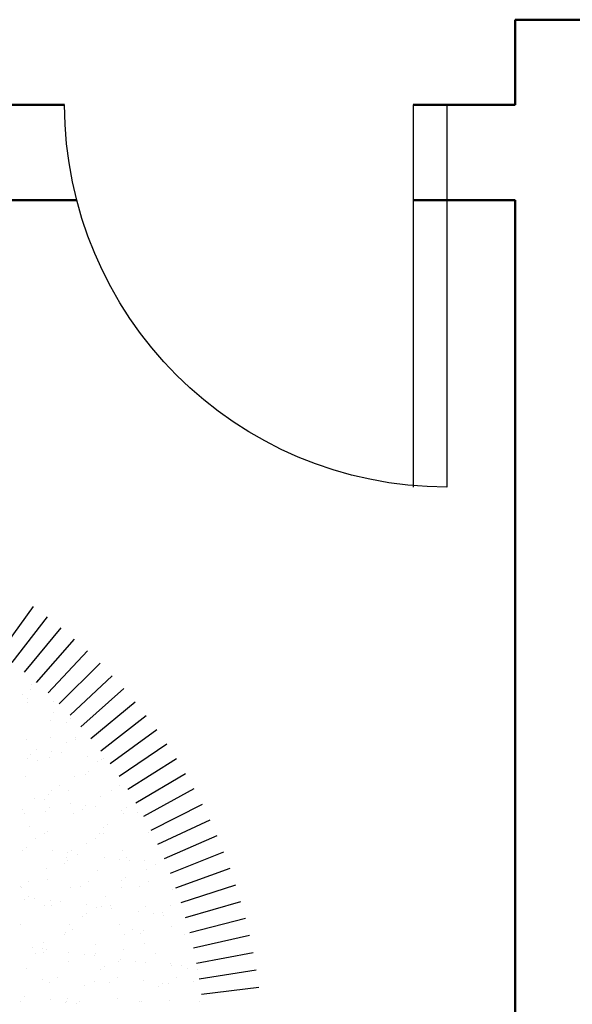
# Model space of a CAD drawing. Units: millimetres. Extents: x -857 to 54106, y -13666 to 13947.
# Tile 16 of 41: x 23479 to 24780, y 5837 to 8154. Entities that reach past the tile are written whole.
import ezdxf

# ---------------------------------------------------------------- set-up
doc = ezdxf.new("R2010")
doc.units = ezdxf.units.MM
for name, color, linetype, lineweight in [('A-DOOR', 1, 'Continuous', 25), ('A-FURN', 21, 'Continuous', 18), ('A-WALL', 7, 'Continuous', 50)]:
    doc.layers.add(name, color=color, linetype=linetype, lineweight=lineweight)
doc.layers.add('A-HT', color=15, linetype='Continuous')

# ---------------------------------------------------------------- blocks, each defined once
blk = doc.blocks.new('*X18')
at = {"color": 0}
for p, q in [((1.1527, 2.5197), (1.1527, 2.5197)), ((1.1551, 2.5078), (1.1551, 2.5078)), ((1.1761, 2.4943), (1.1761, 2.4943)), ((1.0951, 2.4744), (1.0951, 2.4744)), ((1.163, 2.4833), (1.163, 2.4833)), ((1.163, 2.4726), (1.163, 2.4726)), ((1.0963, 2.4457), (1.0963, 2.4457)), ((1.0521, 2.4302), (1.0521, 2.4302)), ((1.0613, 2.4218), (1.0613, 2.4218)), ((1.1027, 2.4263), (1.1027, 2.4263)), ((1.0383, 2.3768), (1.0383, 2.3768)), ((1.0397, 2.3823), (1.0397, 2.3823)), ((1.0608, 2.3689), (1.0608, 2.3689)), ((1.1048, 2.3819), (1.1048, 2.3819)), ((1.1662, 2.3762), (1.1662, 2.3762)), ((1.0745, 2.3422), (1.0745, 2.3422)), ((1.1005, 2.3457), (1.1005, 2.3457)), ((1.1412, 2.351), (1.1412, 2.351)), ((1.1546, 2.3363), (1.1546, 2.3363)), ((0.966, 2.3279), (0.966, 2.3279)), ((0.9708, 2.3251), (0.9708, 2.3251)), ((0.981, 2.3202), (0.981, 2.3202)), ((1.0066, 2.3333), (1.0066, 2.3333)), ((1.1059, 2.33), (1.1059, 2.33)), ((1.1367, 2.3205), (1.1367, 2.3205)), ((1.1638, 2.3279), (1.1638, 2.3279)), ((1.0043, 2.2924), (1.0043, 2.2924)), ((1.0135, 2.284), (1.0135, 2.284)), ((0.9244, 2.2568), (0.9244, 2.2568)), ((1.0414, 2.2805), (1.0414, 2.2805)), ((1.0801, 2.2571), (1.0801, 2.2571)), ((1.1693, 2.2799), (1.1693, 2.2799)), ((0.9455, 2.2434), (0.9455, 2.2434)), ((1.057, 2.2441), (1.057, 2.2441)), ((1.1012, 2.2437), (1.1012, 2.2437)), ((1.109, 2.2336), (1.109, 2.2336)), ((0.974, 2.2287), (0.974, 2.2287)), ((1.0527, 2.2099), (1.0527, 2.2099)), ((1.1206, 2.2189), (1.1206, 2.2189)), ((1.1466, 2.2223), (1.1466, 2.2223)), ((0.8775, 2.1868), (0.8775, 2.1868)), ((0.9067, 2.2002), (0.9067, 2.2002)), ((0.9137, 2.1825), (0.9137, 2.1825)), ((0.9181, 2.1922), (0.9181, 2.1922)), ((0.986, 2.2011), (0.986, 2.2011)), ((1.0121, 2.2046), (1.0121, 2.2046)), ((1.0214, 2.195), (1.0214, 2.195)), ((1.0446, 2.1841), (1.0446, 2.1841)), ((1.1068, 2.1985), (1.1068, 2.1985)), ((1.116, 2.1901), (1.116, 2.1901)), ((1.1725, 2.1835), (1.1725, 2.1835)), ((1.1771, 2.1953), (1.1771, 2.1953)), ((0.9565, 2.1546), (0.9565, 2.1546)), ((0.8492, 2.133), (0.8492, 2.133)), ((0.9648, 2.1316), (0.9648, 2.1316)), ((0.9657, 2.1462), (0.9657, 2.1462)), ((0.9771, 2.1324), (0.9771, 2.1324)), ((1.1122, 2.1373), (1.1122, 2.1373)), ((1.1205, 2.1319), (1.1205, 2.1319)), ((1.1595, 2.1502), (1.1595, 2.1502)), ((0.9859, 2.1182), (0.9859, 2.1182)), ((1.0092, 2.1063), (1.0092, 2.1063)), ((1.1416, 2.1184), (1.1416, 2.1184)), ((0.9169, 2.0861), (0.9169, 2.0861)), ((1.0321, 2.0777), (1.0321, 2.0777)), ((1.0477, 2.0878), (1.0477, 2.0878)), ((1.0582, 2.0812), (1.0582, 2.0812)), ((1.0988, 2.0865), (1.0988, 2.0865)), ((1.1667, 2.0955), (1.1667, 2.0955)), ((1.1756, 2.0872), (1.1756, 2.0872)), ((0.8589, 2.0624), (0.8589, 2.0624)), ((0.8975, 2.06), (0.8975, 2.06)), ((0.9061, 2.0695), (0.9061, 2.0695)), ((0.9236, 2.0635), (0.9236, 2.0635)), ((0.9642, 2.0688), (0.9642, 2.0688)), ((1.059, 2.0607), (1.059, 2.0607)), ((1.0618, 2.0698), (1.0618, 2.0698)), ((1.0682, 2.0523), (1.0682, 2.0523)), ((0.8296, 2.0511), (0.8296, 2.0511)), ((0.8524, 2.0367), (0.8524, 2.0367)), ((0.9803, 2.0361), (0.9803, 2.0361)), ((1.1153, 2.0409), (1.1153, 2.0409)), ((0.8495, 2.0061), (0.8495, 2.0061)), ((0.9087, 2.0168), (0.9087, 2.0168)), ((0.9179, 2.0084), (0.9179, 2.0084)), ((1.0052, 2.0064), (1.0052, 2.0064)), ((1.1117, 2.0124), (1.1117, 2.0124)), ((1.1609, 2.0067), (1.1609, 2.0067)), ((0.785, 1.9849), (0.785, 1.9849)), ((0.8706, 1.9927), (0.8706, 1.9927)), ((0.92, 1.9898), (0.92, 1.9898)), ((1.0263, 1.993), (1.0263, 1.993)), ((1.0509, 1.9915), (1.0509, 1.9915)), ((1.1788, 1.9909), (1.1788, 1.9909)), ((1.182, 1.9932), (1.182, 1.9932)), ((0.9614, 1.9685), (0.9614, 1.9685)), ((1.0782, 1.9544), (1.0782, 1.9544)), ((1.1043, 1.9578), (1.1043, 1.9578)), ((1.1449, 1.9631), (1.1449, 1.9631)), ((1.1614, 1.9668), (1.1614, 1.9668)), ((1.1707, 1.9584), (1.1707, 1.9584)), ((0.7908, 1.944), (0.7908, 1.944)), ((0.8111, 1.9247), (0.8111, 1.9247)), ((0.8555, 1.9403), (0.8555, 1.9403)), ((0.8757, 1.9277), (0.8757, 1.9277)), ((0.9436, 1.9366), (0.9436, 1.9366)), ((0.9465, 1.9443), (0.9465, 1.9443)), ((0.9697, 1.9401), (0.9697, 1.9401)), ((0.9834, 1.9397), (0.9834, 1.9397)), ((1.0103, 1.9454), (1.0103, 1.9454)), ((1.1022, 1.9446), (1.1022, 1.9446)), ((1.1185, 1.9446), (1.1185, 1.9446)), ((0.8091, 1.9189), (0.8091, 1.9189)), ((0.8351, 1.9223), (0.8351, 1.9223)), ((1.0111, 1.9229), (1.0111, 1.9229)), ((1.0204, 1.9145), (1.0204, 1.9145)), ((0.7881, 1.8886), (0.7881, 1.8886)), ((0.8608, 1.879), (0.8608, 1.879)), ((0.8898, 1.8809), (0.8898, 1.8809)), ((0.9232, 1.8935), (0.9232, 1.8935)), ((1.0456, 1.8812), (1.0456, 1.8812)), ((1.054, 1.8951), (1.054, 1.8951)), ((1.0639, 1.8746), (1.0639, 1.8746)), ((1.1819, 1.8945), (1.1819, 1.8945)), ((0.7552, 1.8672), (0.7552, 1.8672)), ((0.8701, 1.8706), (0.8701, 1.8706)), ((0.9109, 1.8675), (0.9109, 1.8675)), ((1.0666, 1.8678), (1.0666, 1.8678)), ((1.1216, 1.8482), (1.1216, 1.8482)), ((0.8587, 1.844), (0.8587, 1.844)), ((0.9136, 1.8307), (0.9136, 1.8307)), ((0.9866, 1.8434), (0.9866, 1.8434)), ((1.0564, 1.822), (1.0564, 1.822)), ((1.1136, 1.829), (1.1136, 1.829)), ((1.1243, 1.831), (1.1243, 1.831)), ((1.1504, 1.8344), (1.1504, 1.8344)), ((0.8311, 1.8188), (0.8311, 1.8188)), ((0.8552, 1.7955), (0.8552, 1.7955)), ((0.8812, 1.799), (0.8812, 1.799)), ((0.9218, 1.8043), (0.9218, 1.8043)), ((0.9263, 1.7971), (0.9263, 1.7971)), ((0.9868, 1.8191), (0.9868, 1.8191)), ((0.9897, 1.8132), (0.9897, 1.8132)), ((1.0158, 1.8167), (1.0158, 1.8167)), ((1.0572, 1.7988), (1.0572, 1.7988)), ((1.1228, 1.8206), (1.1228, 1.8206)), ((1.1425, 1.8194), (1.1425, 1.8194)), ((0.7206, 1.7778), (0.7206, 1.7778)), ((0.7466, 1.7812), (0.7466, 1.7812)), ((0.7632, 1.7869), (0.7632, 1.7869)), ((0.7872, 1.7866), (0.7872, 1.7866)), ((0.7913, 1.7922), (0.7913, 1.7922)), ((0.9633, 1.7851), (0.9633, 1.7851)), ((0.9725, 1.7767), (0.9725, 1.7767)), ((1.1663, 1.7807), (1.1663, 1.7807)), ((0.731, 1.746), (0.731, 1.746)), ((0.7745, 1.7554), (0.7745, 1.7554)), ((0.8618, 1.7477), (0.8618, 1.7477)), ((0.9302, 1.7557), (0.9302, 1.7557)), ((0.9897, 1.747), (0.9897, 1.747)), ((1.0859, 1.756), (1.0859, 1.756)), ((1.1248, 1.7519), (1.1248, 1.7519)), ((0.7956, 1.742), (0.7956, 1.742)), ((0.813, 1.7413), (0.813, 1.7413)), ((0.8222, 1.7328), (0.8222, 1.7328)), ((0.9513, 1.7423), (0.9513, 1.7423)), ((1.016, 1.7368), (1.016, 1.7368)), ((1.107, 1.7426), (1.107, 1.7426)), ((0.7158, 1.6933), (0.7158, 1.6933)), ((0.7944, 1.6959), (0.7944, 1.6959)), ((0.8657, 1.693), (0.8657, 1.693)), ((0.8715, 1.6936), (0.8715, 1.6936)), ((0.9295, 1.7008), (0.9295, 1.7008)), ((1.0272, 1.6939), (1.0272, 1.6939)), ((1.0603, 1.7024), (1.0603, 1.7024)), ((1.0619, 1.6933), (1.0619, 1.6933)), ((1.1025, 1.6986), (1.1025, 1.6986)), ((1.1704, 1.7076), (1.1704, 1.7076)), ((1.1829, 1.6942), (1.1829, 1.6942)), ((1.0358, 1.6899), (1.0358, 1.6899)), ((1.0658, 1.6912), (1.0658, 1.6912))]:
    blk.add_line(p, q, dxfattribs=at)
blk = doc.blocks.new('A$C6796526C')
at = {"layer": 'A-HT'}
for p, q in [((0.1603, 1.2871), (0.0114, 1.2683)), ((0.166, 1.2466), (0.0179, 1.2232)), ((0.173, 1.2064), (0.0257, 1.1783)), ((0.1813, 1.1664), (0.0349, 1.1337)), ((0.1908, 1.1267), (0.0456, 1.0894)), ((0.2016, 1.0873), (0.0576, 1.0455)), ((0.2136, 1.0483), (0.071, 1.0019)), ((0.2269, 1.0096), (0.0857, 0.9588)), ((0.2413, 0.9714), (0.1018, 0.9162)), ((0.2569, 0.9337), (0.1193, 0.8741)), ((0.2737, 0.8965), (0.138, 0.8326)), ((0.2917, 0.8598), (0.158, 0.7917)), ((0.3108, 0.8237), (0.1794, 0.7515)), ((0.331, 0.7882), (0.2019, 0.7119)), ((0.3524, 0.7534), (0.2257, 0.6731)), ((0.3748, 0.7193), (0.2507, 0.635)), ((0.3983, 0.6859), (0.2769, 0.5977)), ((0.4228, 0.6532), (0.3043, 0.5613)), ((0.4483, 0.6213), (0.3328, 0.5257)), ((0.4749, 0.5903), (0.3623, 0.4911)), ((0.5023, 0.5601), (0.393, 0.4574)), ((0.5308, 0.5308), (0.4247, 0.4247)), ((0.5601, 0.5023), (0.4574, 0.393)), ((0.5903, 0.4749), (0.4911, 0.3623)), ((0.6213, 0.4483), (0.5257, 0.3328)), ((0.6532, 0.4228), (0.5613, 0.3043)), ((0.6859, 0.3983), (0.5977, 0.2769))]:
    blk.add_line(p, q, dxfattribs=at)
at = {"layer": 'A-HT', "extrusion": (0, 0, -1), "zscale": -1, "rotation": 180}
blk.add_blockref('*X18', (0.55, 3), dxfattribs=at)
blk = doc.blocks.new('DOOR-900')
blk.add_line((11417.3, 9811.5), (12317.3, 9811.5))
blk.add_arc((11417.3, 9811.5), 900, 0, 90)

msp = doc.modelspace()

# ---------------------------------------------------------------- linework, layer by layer
at = {"layer": 'A-DOOR'}
msp.add_line((24404.957, 7954.231), (24404.957, 7054.231), dxfattribs=at)
at = {"layer": 'A-WALL'}
for p, q in [((24645.079, 8154.231), (24645.079, 7954.231)), ((24645.079, 8154.231), (24870.079, 8154.231)), ((23584.957, 7954.231), (23445.079, 7954.231)), ((24645.079, 7954.231), (24404.957, 7954.231)), ((21245.079, 7729.231), (23613.536, 7729.231)), ((24404.957, 7729.231), (24645.079, 7729.231)), ((24645.079, 7729.231), (24645.079, 4129.231))]:
    msp.add_line(p, q, dxfattribs=at)

# ---------------------------------------------------------------- block references
at = {"layer": 'A-DOOR', "extrusion": (0, 0, -1), "zscale": -1, "rotation": 269.9999999999998}
msp.add_blockref('DOOR-900', (-34296.438, 19371.511), dxfattribs=at)
at = {"layer": 'A-FURN', "xscale": 903.6084929786902, "yscale": 903.6084929786902, "zscale": 903.6084929786902, "rotation": 179.9999999999989}
msp.add_blockref('A$C6796526C', (24051.97, 7023.692), dxfattribs=at)

doc.saveas('drawing.dxf')
